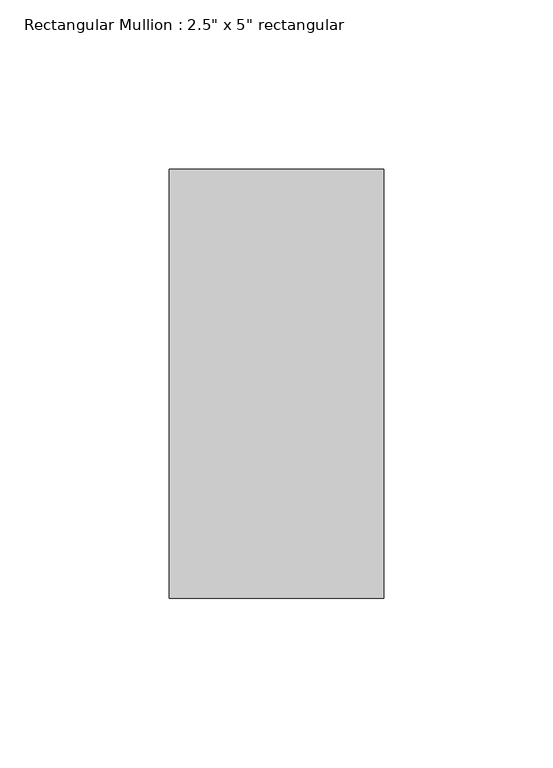
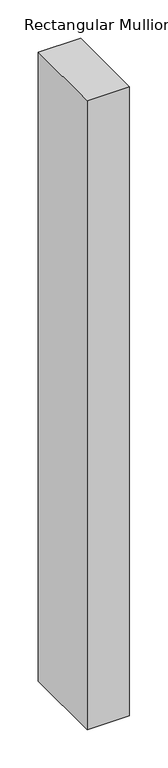
"""IFC4 building model written with IfcOpenShell, lengths in millimetres: member geometry."""

from ifc_helpers import new_model, si_unit, frame, origin, place, context, project, spatial, polyline, outline, extrude, source, transform, mapped, element, save


def member_e156fde9(model_context):
    return source(origin(), model_context, "Body", "SweptSolid", [
        extrude(outline(polyline([(0.0, 63.5), (0.0, -63.5), (-63.5, -63.5), (-63.5, 63.5), (0.0, 63.5)])), frame((0.0, 0.0, -1001.0022263), z_axis=(0.0, 0.0, 1.0), x_axis=(1.0, 0.0, 0.0)), (0.0, 0.0, 1.0), 1001.0022263),
    ])


if __name__ == "__main__":
    model = new_model("IFC4")
    model_context = context("Model", 3, world=origin())
    ifc_project = project(units=[si_unit("LENGTHUNIT", "METRE", prefix="MILLI")], contexts=[model_context])
    site = spatial("IfcSite", under=ifc_project)
    building = spatial("IfcBuilding", under=site)
    placement = place(None, origin())
    member_shape = member_e156fde9(model_context)
    element("IfcMember", 1, ObjectType="Rectangular Mullion : 2.5\" x 5\" rectangular", at=placement, inside=building, context=model_context, shape_type="MappedRepresentation", body=[
        mapped(member_shape, transform((0.0, 0.0, 0.0), x_axis=(1.0, 0.0, 0.0), y_axis=(0.0, 1.0, 0.0), z_axis=(0.0, 0.0, 1.0))),
    ])
    save(model, "model.ifc")

# Revit data of these elements
# Type "Rectangular Mullion : 2.5\" x 5\" rectangular"
#   built-in parameter 1007304 = 0.416667 (stored number, unit not read)
#   built-in parameter 1007301 = 0.104167 (stored number, unit not read)
#   built-in parameter 1007300 = 0.104167 (stored number, unit not read)
# Element 1 (IfcMember, "Rectangular Mullion : 2.5\" x 5\" rectangular")
#   Materials on its faces: "Aluminum"
# Materials
#   "Aluminum": class "Metal", colour RGB 247 247 247, transparency 0, Description = "Aluminum 6061", Cost = 0
